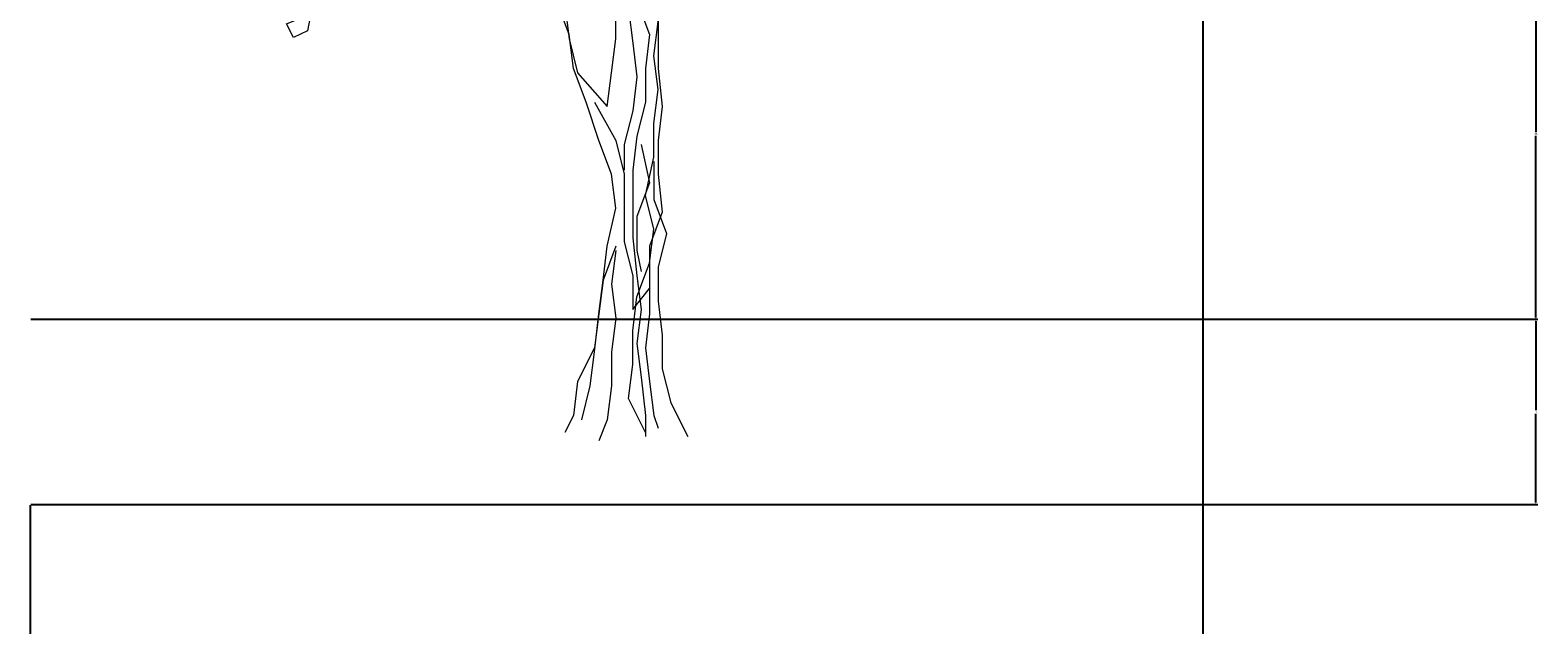
# Model space of a CAD drawing. Units: inches. Extents: x 1770 to 2988, y 1161 to 3221.
# Tile 38 of 44: x 2655 to 2802, y 2693 to 2750. Entities that reach past the tile are written whole.
import ezdxf

# ---------------------------------------------------------------- set-up
doc = ezdxf.new("R2010")
doc.units = ezdxf.units.IN
for name, color, linetype, lineweight in [('A-ANNO-DIMS', 2, 'Continuous', 18), ('A-ANNO-TTLB', 7, 'Continuous', 25), ('trees1', 250, 'Continuous', 13)]:
    doc.layers.add(name, color=color, linetype=linetype, lineweight=lineweight)
doc.styles.get("Standard").update_dxf_attribs({"font": 'arial.ttf'})
doc.dimstyles.get("Standard").update_dxf_attribs({"dimtxt": 0.18, "dimasz": 0.18, "dimexe": 0.18, "dimexo": 0.0625, "dimgap": 0.09, "dimtad": 0, "dimtih": 1, "dimtoh": 1, "dimdec": 4, "dimzin": 0, "dimdsep": 46, "dimtxsty": 'Standard', "dimcen": 0.09, "dimadec": 0, "dimazin": 0, "dimtfac": 1, "dimtdec": 4, "dimtofl": 0, "dimtmove": 0, "dimatfit": 3, "dimfxl": 1, "dimtolj": 1, "dimtzin": 0, "dimarcsym": 0})

# ---------------------------------------------------------------- blocks, each defined once
blk = doc.blocks.new('tree342')
at = {"color": 0}
for p, q in [((-110.8, 612.1), (-110.8, 716.3)), ((-189, 664.2), (-182.5, 612.1)), ((-182.5, 612.1), (-169.4, 560)), ((-117.3, 560), (-110.8, 612.1)), ((-169.4, 560), (-123.8, 507.9)), ((-123.8, 507.9), (-117.3, 560))]:
    blk.add_line(p, q, dxfattribs=at)
for points in [[(39.1, 1243.8), (-13, 1204.7), (-45.6, 1152.6), (-45.6, 1100.5), (-32.6, 1048.4), (-39.1, 996.3), (-39.1, 944.2), (-45.6, 892.1), (-65.2, 833.5), (-58.6, 774.9), (-78.2, 722.8), (-78.2, 670.7), (-58.6, 618.6), (-65.2, 566.5), (-65.2, 514.4), (-78.2, 462.3), (-84.7, 410.2), (-84.7, 306.1), (-78.2, 247.5), (-71.7, 195.4), (-78.2, 143.3), (-71.7, 91.2), (-65.2, 32.6), (-65.2, 0)], [(293.2, 1139.6), (273.7, 1087.5), (241.1, 1035.4), (208.5, 983.3), (156.4, 937.7), (110.8, 885.6), (71.7, 833.5), (32.6, 781.4), (-13, 729.3), (-45.6, 677.2), (-45.6, 566.5), (-39.1, 507.9), (-45.6, 455.8), (-45.6, 403.7), (-39.1, 345.1), (-58.6, 293), (-58.6, 188.8), (-65.2, 136.7), (-58.6, 84.7), (-52.1, 32.6), (-45.6, 13)], [(-65.2, 6.5), (-91.2, 58.6), (-84.7, 110.7), (-84.7, 162.8), (-78.2, 214.9), (-58.6, 267), (-52.1, 319.1), (-65.2, 371.2), (-52.1, 429.8), (-52.1, 481.9), (-45.6, 534), (-52.1, 586.1), (-45.6, 638.2), (-58.6, 690.3), (-39.1, 742.4), (13, 774.9), (52.1, 827), (97.7, 879.1), (117.3, 931.2), (169.4, 957.2), (221.6, 1002.8), (247.6, 1054.9), (260.6, 1074.5)], [(-136.8, 1028.9), (-91.2, 976.8), (-84.7, 924.7), (-71.7, 872.6), (-71.7, 820.5), (-78.2, 768.4), (-78.2, 709.8), (-91.2, 657.7), (-84.7, 605.6), (-78.2, 553.5), (-84.7, 501.4), (-97.7, 449.3), (-97.7, 410.2)], [(-162.9, 26), (-149.9, 78.1), (-143.4, 130.2), (-136.8, 188.8), (-130.3, 240.9), (-123.8, 293), (-110.8, 351.6), (-117.3, 403.7), (-136.8, 455.8), (-156.4, 514.4), (-175.9, 566.5), (-182.5, 618.6), (-202, 670.7), (-208.5, 722.8), (-234.6, 774.9), (-254.1, 820.5)], [(-580.9, 646.1), (-585.2, 624.6), (-606.7, 613.9), (-617.4, 635.4), (-596, 644), (-576.6, 646.1)], [(-143.4, 514.4), (-110.8, 455.8), (-97.7, 403.7), (-97.7, 299.5), (-84.7, 247.5), (-84.7, 195.4), (-58.6, 227.9)], [(-71.7, 449.3), (-58.6, 390.7), (-78.2, 338.6), (-78.2, 286.5), (-71.7, 254)], [(-52.1, 423.3), (-52.1, 364.7), (-32.6, 312.6), (-45.6, 260.5), (-45.6, 208.4), (-39.1, 156.3), (-39.1, 104.2), (-26.1, 52.1), (0, 0)], [(-110.8, 293), (-130.3, 240.9), (-136.8, 188.8), (-143.4, 136.7), (-169.4, 84.7), (-175.9, 32.6), (-189, 6.5)], [(-110.8, 286.5), (-117.3, 234.4), (-110.8, 182.3), (-117.3, 130.2), (-117.3, 78.1), (-123.8, 26), (-136.8, -6.5)]]:
    blk.add_lwpolyline(points, dxfattribs=at)
blk = doc.blocks.new('*D93')
at = {"layer": 'A-ANNO-DIMS', "color": 0, "lineweight": -2, "transparency": 16777216}
for p, q in [((2181.44, 2704.23), (2181.44, 2545.88)), ((2655.44, 2704.23), (2655.44, 2545.88)), ((2181.62, 2546.06), (2418.15, 2546.06)), ((2655.26, 2546.06), (2418.74, 2546.06))]:
    blk.add_line(p, q, dxfattribs=at)
at = {"layer": 'A-ANNO-DIMS', "color": 0, "transparency": 16777216}
for points in [[(2181.62, 2546.09), (2181.62, 2546.03), (2181.44, 2546.06)], [(2655.26, 2546.09), (2655.26, 2546.03), (2655.44, 2546.06)]]:
    blk.add_solid(points, dxfattribs=at)
at = {"layer": 'Defpoints', "color": 0, "transparency": 16777216}
for p in [(2181.44, 2704.3), (2655.44, 2704.3), (2655.44, 2546.06)]:
    blk.add_point(p, dxfattribs=at)
at = {"layer": 'A-ANNO-DIMS', "color": 0, "transparency": 16777216, "insert": (2418.44, 2546.06), "char_height": 0.18, "attachment_point": 5}
blk.add_mtext('\\A1;474', dxfattribs=at)
blk = doc.blocks.new('*D95')
at = {"layer": 'A-ANNO-DIMS', "color": 0, "lineweight": -2, "transparency": 16777216}
for p, q in [((2655.51, 2722.3), (2801.91, 2722.3)), ((2801.73, 2722.12), (2801.73, 2713.48)), ((2801.73, 2704.48), (2801.73, 2713.11)), ((2655.51, 2704.3), (2801.91, 2704.3))]:
    blk.add_line(p, q, dxfattribs=at)
at = {"layer": 'A-ANNO-DIMS', "color": 0, "transparency": 16777216}
for points in [[(2801.7, 2722.12), (2801.76, 2722.12), (2801.73, 2722.3)], [(2801.7, 2704.48), (2801.76, 2704.48), (2801.73, 2704.3)]]:
    blk.add_solid(points, dxfattribs=at)
at = {"layer": 'Defpoints', "color": 0, "transparency": 16777216}
for p in [(2655.44, 2722.3), (2801.73, 2722.3), (2655.44, 2704.3)]:
    blk.add_point(p, dxfattribs=at)
at = {"layer": 'A-ANNO-DIMS', "color": 0, "transparency": 16777216, "insert": (2801.73, 2713.3), "char_height": 0.18, "attachment_point": 5}
blk.add_mtext('\\A1;18', dxfattribs=at)
blk = doc.blocks.new('*D96')
at = {"layer": 'A-ANNO-DIMS', "color": 0, "lineweight": -2, "transparency": 16777216}
for p, q in [((2620.11, 2758.3), (2801.91, 2758.3)), ((2801.73, 2758.12), (2801.73, 2740.48)), ((2801.73, 2722.48), (2801.73, 2740.11)), ((2655.51, 2722.3), (2801.91, 2722.3))]:
    blk.add_line(p, q, dxfattribs=at)
at = {"layer": 'A-ANNO-DIMS', "color": 0, "transparency": 16777216}
for points in [[(2801.7, 2758.12), (2801.76, 2758.12), (2801.73, 2758.3)], [(2801.7, 2722.48), (2801.76, 2722.48), (2801.73, 2722.3)]]:
    blk.add_solid(points, dxfattribs=at)
at = {"layer": 'Defpoints', "color": 0, "transparency": 16777216}
for p in [(2620.05, 2758.3), (2801.73, 2758.3), (2655.44, 2722.3)]:
    blk.add_point(p, dxfattribs=at)
at = {"layer": 'A-ANNO-DIMS', "color": 0, "transparency": 16777216, "insert": (2801.73, 2740.3), "char_height": 0.18, "attachment_point": 5}
blk.add_mtext('\\A1;36', dxfattribs=at)

msp = doc.modelspace()

# ---------------------------------------------------------------- linework, layer by layer
at = {"layer": 'A-ANNO-TTLB'}
msp.add_lwpolyline([(2073.6202, 3129.9468), (2769.3644, 3129.9468), (2769.3644, 2546.8952), (2073.6202, 2546.8952)], close=True, dxfattribs=at)

# ---------------------------------------------------------------- block references
at = {"layer": 'trees1', "xscale": 0.063143750371755, "yscale": 0.063143750371755, "zscale": 0.063143750371755}
msp.add_blockref('tree342', (2719.3275, 2710.8976), dxfattribs=at)

# ---------------------------------------------------------------- dimensions: what is measured, and where the dimension line sits
at = {"layer": 'A-ANNO-DIMS'}
for base, p1, p2, picture, middle in [((2801.7346, 2758.2969), (2655.443, 2722.2969), (2620.0508, 2758.2969), '*D96', (2801.7346, 2740.2969)), ((2801.7346, 2722.2969), (2655.443, 2704.2969), (2655.443, 2722.2969), '*D95', (2801.7346, 2713.2969))]:
    dim = msp.add_linear_dim(base=base, p1=p1, p2=p2, angle=90, dimstyle='Standard', override={"dimdec": 0, "dimlfac": 1, "dimrnd": 0, "dimzin": 0, "dimdsep": 46, "dimlunit": 2}, dxfattribs=at)
    dim.commit()
    dim.dimension.update_dxf_attribs({"geometry": picture, "text_midpoint": middle})
dim = msp.add_linear_dim(base=(2655.443, 2546.0579), p1=(2181.443, 2704.2969), p2=(2655.443, 2704.2969), dimstyle='Standard', override={"dimdec": 0, "dimlfac": 1, "dimrnd": 0, "dimzin": 0, "dimdsep": 46, "dimlunit": 2}, dxfattribs=at)
dim.commit()
dim.dimension.update_dxf_attribs({"geometry": '*D93', "text_midpoint": (2418.443, 2546.0579)})

doc.saveas('drawing.dxf')
